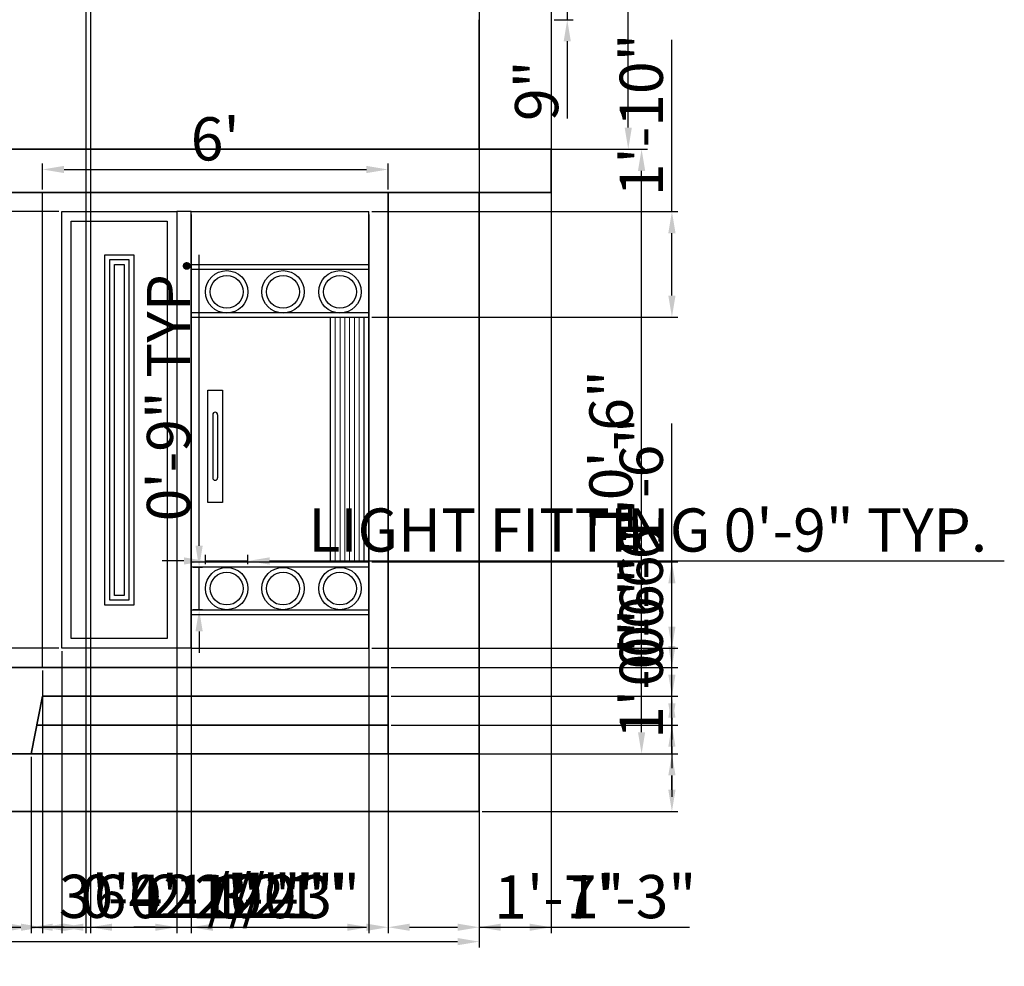
# Model space of a CAD drawing. Units: inches. Extents: x 3297 to 3846, y 520 to 959.
# Tile 3 of 5: x 3641 to 3846, y 520 to 717. Entities that reach past the tile are written whole.
import ezdxf

# ---------------------------------------------------------------- set-up
doc = ezdxf.new("R2010")
doc.units = ezdxf.units.IN
for name, color, linetype, lineweight in [('A-ANNO-DIMS', 2, 'Continuous', 18), ('A-DOOR', 4, 'Continuous', 25), ('A-ELEV', 7, 'Continuous', 35), ('A-ELEV-PATT', 8, 'Continuous', 13)]:
    doc.layers.add(name, color=color, linetype=linetype, lineweight=lineweight)
doc.styles.get("Standard").update_dxf_attribs({"font": 'arial.ttf'})
doc.dimstyles.new('ISO-25', dxfattribs={"dimtxt": 9, "dimasz": 4.5, "dimexe": 1.25, "dimexo": 0.625, "dimtad": 1, "dimdec": 0, "dimlunit": 3, "dimtxsty": 'Standard', "dimcen": 2.5, "dimadec": 0, "dimazin": 0, "dimtfac": 1, "dimtdec": 0, "dimtmove": 0, "dimatfit": 3, "dimfxl": 1, "dimarcsym": 0})

# ---------------------------------------------------------------- blocks, each defined once
blk = doc.blocks.new('*D1')
at = {"layer": 'A-ANNO-DIMS', "color": 0, "lineweight": -2, "transparency": 16777216}
for p, q in [((3737.69, 690.24), (3772.14, 690.24)), ((3770.89, 568.74), (3770.89, 685.74)), ((3737.69, 564.24), (3772.14, 564.24))]:
    blk.add_line(p, q, dxfattribs=at)
at = {"layer": 'A-ANNO-DIMS', "color": 0, "transparency": 16777216}
for points in [[(3770.14, 685.74), (3771.64, 685.74), (3770.89, 690.24)], [(3770.14, 568.74), (3771.64, 568.74), (3770.89, 564.24)]]:
    blk.add_solid(points, dxfattribs=at)
at = {"layer": 'Defpoints', "color": 0, "transparency": 16777216}
for p in [(3737.06, 690.24), (3770.89, 690.24), (3737.06, 564.24)]:
    blk.add_point(p, dxfattribs=at)
at = {"layer": 'A-ANNO-DIMS', "color": 0, "transparency": 16777216, "insert": (3765.67, 627.24), "char_height": 9, "attachment_point": 5, "rotation": 90}
blk.add_mtext('10\'-6"', dxfattribs=at)
blk = doc.blocks.new('*D2')
at = {"layer": 'A-ANNO-DIMS', "color": 0, "lineweight": -2, "transparency": 16777216}
for p, q in [((3752.69, 828.24), (3769.36, 828.24)), ((3768.11, 694.74), (3768.11, 823.74)), ((3752.69, 690.24), (3769.36, 690.24))]:
    blk.add_line(p, q, dxfattribs=at)
at = {"layer": 'A-ANNO-DIMS', "color": 0, "transparency": 16777216}
for points in [[(3767.36, 823.74), (3768.86, 823.74), (3768.11, 828.24)], [(3767.36, 694.74), (3768.86, 694.74), (3768.11, 690.24)]]:
    blk.add_solid(points, dxfattribs=at)
at = {"layer": 'Defpoints', "color": 0, "transparency": 16777216}
for p in [(3752.06, 828.24), (3768.11, 828.24), (3752.06, 690.24)]:
    blk.add_point(p, dxfattribs=at)
at = {"layer": 'A-ANNO-DIMS', "color": 0, "transparency": 16777216, "insert": (3762.89, 759.24), "char_height": 9, "attachment_point": 5, "rotation": 90}
blk.add_mtext('11\'-6"', dxfattribs=at)
blk = doc.blocks.new('*D7')
at = {"layer": 'A-ANNO-DIMS', "color": 0, "lineweight": -2, "transparency": 16777216}
for p, q in [((3332.06, 551.62), (3332.06, 523.84)), ((3737.06, 551.62), (3737.06, 523.84)), ((3336.56, 525.09), (3732.56, 525.09))]:
    blk.add_line(p, q, dxfattribs=at)
at = {"layer": 'A-ANNO-DIMS', "color": 0, "transparency": 16777216}
for points in [[(3336.56, 525.84), (3336.56, 524.34), (3332.06, 525.09)], [(3732.56, 525.84), (3732.56, 524.34), (3737.06, 525.09)]]:
    blk.add_solid(points, dxfattribs=at)
at = {"layer": 'Defpoints', "color": 0, "transparency": 16777216}
for p in [(3332.06, 552.24), (3737.06, 552.24), (3737.06, 525.09)]:
    blk.add_point(p, dxfattribs=at)
at = {"layer": 'A-ANNO-DIMS', "color": 0, "transparency": 16777216, "insert": (3534.56, 530.31), "char_height": 9, "attachment_point": 5}
blk.add_mtext('33\'-9"', dxfattribs=at)
blk = doc.blocks.new('*D11')
at = {"layer": 'A-ANNO-DIMS', "color": 0, "lineweight": -2, "transparency": 16777216}
for p, q in [((3646.06, 681.87), (3646.06, 687.27)), ((3650.56, 686.02), (3713.56, 686.02)), ((3718.06, 681.87), (3718.06, 687.27))]:
    blk.add_line(p, q, dxfattribs=at)
at = {"layer": 'A-ANNO-DIMS', "color": 0, "transparency": 16777216}
for points in [[(3650.56, 686.77), (3650.56, 685.27), (3646.06, 686.02)], [(3713.56, 686.77), (3713.56, 685.27), (3718.06, 686.02)]]:
    blk.add_solid(points, dxfattribs=at)
at = {"layer": 'Defpoints', "color": 0, "transparency": 16777216}
for p in [(3718.06, 686.02), (3646.06, 681.24), (3718.06, 681.24)]:
    blk.add_point(p, dxfattribs=at)
at = {"layer": 'A-ANNO-DIMS', "color": 0, "transparency": 16777216, "insert": (3682.06, 691.24), "char_height": 9, "attachment_point": 5}
blk.add_mtext("6'", dxfattribs=at)
blk = doc.blocks.new('*D17')
at = {"layer": 'A-ANNO-DIMS', "color": 0, "lineweight": -2, "transparency": 16777216}
for p, q in [((3755.4, 730.74), (3755.4, 735.24)), ((3752.69, 726.24), (3756.65, 726.24)), ((3755.4, 726.24), (3755.4, 717.24)), ((3752.69, 717.24), (3756.65, 717.24)), ((3755.4, 712.74), (3755.4, 696.65))]:
    blk.add_line(p, q, dxfattribs=at)
at = {"layer": 'A-ANNO-DIMS', "color": 0, "transparency": 16777216}
for points in [[(3754.65, 730.74), (3756.15, 730.74), (3755.4, 726.24)], [(3754.65, 712.74), (3756.15, 712.74), (3755.4, 717.24)]]:
    blk.add_solid(points, dxfattribs=at)
at = {"layer": 'Defpoints', "color": 0, "transparency": 16777216}
for p in [(3752.06, 726.24), (3752.06, 717.24), (3755.4, 717.24)]:
    blk.add_point(p, dxfattribs=at)
at = {"layer": 'A-ANNO-DIMS', "color": 0, "transparency": 16777216, "insert": (3750.18, 702.44), "char_height": 9, "attachment_point": 5, "rotation": 90}
blk.add_mtext('9"', dxfattribs=at)
blk = doc.blocks.new('LIGHT-ROUND')
for radius in [4.42, 3.42]:
    blk.add_circle((3684.44, 660.52), radius)
blk = doc.blocks.new('*D25')
at = {"layer": 'A-ANNO-DIMS', "color": 0, "lineweight": -2, "transparency": 16777216}
for p, q in [((3680.01, 603.73), (3680.01, 605.68)), ((3688.86, 603.73), (3688.86, 605.68)), ((3675.51, 604.43), (3671.01, 604.43)), ((3680.01, 604.43), (3688.86, 604.43)), ((3693.36, 604.43), (3846.47, 604.43))]:
    blk.add_line(p, q, dxfattribs=at)
at = {"layer": 'A-ANNO-DIMS', "color": 0, "transparency": 16777216}
for points in [[(3675.51, 605.18), (3675.51, 603.68), (3680.01, 604.43)], [(3693.36, 605.18), (3693.36, 603.68), (3688.86, 604.43)]]:
    blk.add_solid(points, dxfattribs=at)
at = {"layer": 'Defpoints', "color": 0, "transparency": 16777216}
for p in [(3688.86, 604.43), (3680.01, 603.1), (3688.86, 603.1)]:
    blk.add_point(p, dxfattribs=at)
at = {"layer": 'A-ANNO-DIMS', "color": 0, "transparency": 16777216, "insert": (3772.17, 609.71), "char_height": 9, "attachment_point": 5}
blk.add_mtext('LIGHT FITTING 0\'-9" TYP.', dxfattribs=at)
blk = doc.blocks.new('*D26')
at = {"layer": 'A-ANNO-DIMS', "color": 0, "lineweight": -2, "transparency": 16777216}
for p, q in [((3678.69, 607.6), (3678.69, 668.21)), ((3679.39, 603.1), (3677.44, 603.1)), ((3678.69, 594.25), (3678.69, 603.1)), ((3679.39, 594.25), (3677.44, 594.25)), ((3678.69, 589.75), (3678.69, 585.25))]:
    blk.add_line(p, q, dxfattribs=at)
at = {"layer": 'A-ANNO-DIMS', "color": 0, "transparency": 16777216}
for points in [[(3677.94, 607.6), (3679.44, 607.6), (3678.69, 603.1)], [(3677.94, 589.75), (3679.44, 589.75), (3678.69, 594.25)]]:
    blk.add_solid(points, dxfattribs=at)
at = {"layer": 'Defpoints', "color": 0, "transparency": 16777216}
for p in [(3678.69, 603.1), (3680.01, 603.1), (3680.01, 594.25)]:
    blk.add_point(p, dxfattribs=at)
at = {"layer": 'A-ANNO-DIMS', "color": 0, "transparency": 16777216, "insert": (3673.47, 640.16), "char_height": 9, "attachment_point": 5, "rotation": 90}
blk.add_mtext('0\'-9" TYP.', dxfattribs=at)
blk = doc.blocks.new('*D41')
at = {"layer": 'A-ANNO-DIMS', "color": 0, "lineweight": -2, "transparency": 16777216}
for p, q in [((3655.06, 882.62), (3655.06, 526.84)), ((3656.06, 882.62), (3656.06, 526.84)), ((3650.56, 528.09), (3646.06, 528.09)), ((3655.06, 528.09), (3656.06, 528.09)), ((3660.56, 528.09), (3690.24, 528.09))]:
    blk.add_line(p, q, dxfattribs=at)
at = {"layer": 'A-ANNO-DIMS', "color": 0, "transparency": 16777216}
for points in [[(3650.56, 528.84), (3650.56, 527.34), (3655.06, 528.09)], [(3660.56, 528.84), (3660.56, 527.34), (3656.06, 528.09)]]:
    blk.add_solid(points, dxfattribs=at)
at = {"layer": 'Defpoints', "color": 0, "transparency": 16777216}
for p in [(3655.06, 883.24), (3656.06, 883.24), (3656.06, 528.09)]:
    blk.add_point(p, dxfattribs=at)
at = {"layer": 'A-ANNO-DIMS', "color": 0, "transparency": 16777216, "insert": (3677.65, 533.31), "char_height": 9, "attachment_point": 5}
blk.add_mtext('0\'-1"', dxfattribs=at)
blk = doc.blocks.new('*D45')
at = {"layer": 'A-ANNO-DIMS', "color": 0, "lineweight": -2, "transparency": 16777216}
for p, q in [((3737.06, 816.62), (3737.06, 526.84)), ((3752.06, 816.62), (3752.06, 526.84)), ((3741.56, 528.09), (3747.56, 528.09)), ((3752.06, 528.09), (3780.89, 528.09))]:
    blk.add_line(p, q, dxfattribs=at)
at = {"layer": 'A-ANNO-DIMS', "color": 0, "transparency": 16777216}
for points in [[(3741.56, 528.84), (3741.56, 527.34), (3737.06, 528.09)], [(3747.56, 528.84), (3747.56, 527.34), (3752.06, 528.09)]]:
    blk.add_solid(points, dxfattribs=at)
at = {"layer": 'Defpoints', "color": 0, "transparency": 16777216}
for p in [(3737.06, 817.24), (3752.06, 817.24), (3752.06, 528.09)]:
    blk.add_point(p, dxfattribs=at)
at = {"layer": 'A-ANNO-DIMS', "color": 0, "transparency": 16777216, "insert": (3768.73, 533.31), "char_height": 9, "attachment_point": 5}
blk.add_mtext('1\'-3"', dxfattribs=at)
blk = doc.blocks.new('*D46')
at = {"layer": 'A-ANNO-DIMS', "color": 0, "lineweight": -2, "transparency": 16777216}
for p, q in [((3777.21, 564.24), (3777.21, 593.07)), ((3737.69, 564.24), (3778.46, 564.24)), ((3777.21, 556.74), (3777.21, 559.74)), ((3737.69, 552.24), (3778.46, 552.24))]:
    blk.add_line(p, q, dxfattribs=at)
at = {"layer": 'A-ANNO-DIMS', "color": 0, "transparency": 16777216}
for points in [[(3776.46, 559.74), (3777.96, 559.74), (3777.21, 564.24)], [(3776.46, 556.74), (3777.96, 556.74), (3777.21, 552.24)]]:
    blk.add_solid(points, dxfattribs=at)
at = {"layer": 'Defpoints', "color": 0, "transparency": 16777216}
for p in [(3737.06, 564.24), (3777.21, 564.24), (3737.06, 552.24)]:
    blk.add_point(p, dxfattribs=at)
at = {"layer": 'A-ANNO-DIMS', "color": 0, "transparency": 16777216, "insert": (3771.99, 580.9), "char_height": 9, "attachment_point": 5, "rotation": 90}
blk.add_mtext('1\'-0"', dxfattribs=at)
blk = doc.blocks.new('*D47')
at = {"layer": 'A-ANNO-DIMS', "color": 0, "lineweight": -2, "transparency": 16777216}
for p, q in [((3777.21, 574.74), (3777.21, 604.42)), ((3718.69, 570.24), (3778.46, 570.24)), ((3777.21, 564.24), (3777.21, 570.24)), ((3718.69, 564.24), (3778.46, 564.24)), ((3777.21, 559.74), (3777.21, 555.24))]:
    blk.add_line(p, q, dxfattribs=at)
at = {"layer": 'A-ANNO-DIMS', "color": 0, "transparency": 16777216}
for points in [[(3776.46, 574.74), (3777.96, 574.74), (3777.21, 570.24)], [(3776.46, 559.74), (3777.96, 559.74), (3777.21, 564.24)]]:
    blk.add_solid(points, dxfattribs=at)
at = {"layer": 'Defpoints', "color": 0, "transparency": 16777216}
for p in [(3718.06, 570.24), (3777.21, 570.24), (3718.06, 564.24)]:
    blk.add_point(p, dxfattribs=at)
at = {"layer": 'A-ANNO-DIMS', "color": 0, "transparency": 16777216, "insert": (3771.99, 591.83), "char_height": 9, "attachment_point": 5, "rotation": 90}
blk.add_mtext('0\'-6"', dxfattribs=at)
blk = doc.blocks.new('*D48')
at = {"layer": 'A-ANNO-DIMS', "color": 0, "lineweight": -2, "transparency": 16777216}
for p, q in [((3777.21, 580.74), (3777.21, 610.42)), ((3718.69, 576.24), (3778.46, 576.24)), ((3777.21, 570.24), (3777.21, 576.24)), ((3718.69, 570.24), (3778.46, 570.24)), ((3777.21, 565.74), (3777.21, 561.24))]:
    blk.add_line(p, q, dxfattribs=at)
at = {"layer": 'A-ANNO-DIMS', "color": 0, "transparency": 16777216}
for points in [[(3776.46, 580.74), (3777.96, 580.74), (3777.21, 576.24)], [(3776.46, 565.74), (3777.96, 565.74), (3777.21, 570.24)]]:
    blk.add_solid(points, dxfattribs=at)
at = {"layer": 'Defpoints', "color": 0, "transparency": 16777216}
for p in [(3718.06, 576.24), (3777.21, 576.24), (3718.06, 570.24)]:
    blk.add_point(p, dxfattribs=at)
at = {"layer": 'A-ANNO-DIMS', "color": 0, "transparency": 16777216, "insert": (3771.99, 597.83), "char_height": 9, "attachment_point": 5, "rotation": 90}
blk.add_mtext('0\'-6"', dxfattribs=at)
blk = doc.blocks.new('*D49')
at = {"layer": 'A-ANNO-DIMS', "color": 0, "lineweight": -2, "transparency": 16777216}
for p, q in [((3777.21, 586.74), (3777.21, 616.42)), ((3718.69, 582.24), (3778.46, 582.24)), ((3777.21, 576.24), (3777.21, 582.24)), ((3718.69, 576.24), (3778.46, 576.24)), ((3777.21, 571.74), (3777.21, 567.24))]:
    blk.add_line(p, q, dxfattribs=at)
at = {"layer": 'A-ANNO-DIMS', "color": 0, "transparency": 16777216}
for points in [[(3776.46, 586.74), (3777.96, 586.74), (3777.21, 582.24)], [(3776.46, 571.74), (3777.96, 571.74), (3777.21, 576.24)]]:
    blk.add_solid(points, dxfattribs=at)
at = {"layer": 'Defpoints', "color": 0, "transparency": 16777216}
for p in [(3718.06, 582.24), (3777.21, 582.24), (3718.06, 576.24)]:
    blk.add_point(p, dxfattribs=at)
at = {"layer": 'A-ANNO-DIMS', "color": 0, "transparency": 16777216, "insert": (3771.99, 603.83), "char_height": 9, "attachment_point": 5, "rotation": 90}
blk.add_mtext('0\'-6"', dxfattribs=at)
blk = doc.blocks.new('*D50')
at = {"layer": 'A-ANNO-DIMS', "color": 0, "lineweight": -2, "transparency": 16777216}
for p, q in [((3643.69, 563.62), (3643.69, 526.84)), ((3718.06, 563.62), (3718.06, 526.84)), ((3648.19, 528.09), (3713.56, 528.09))]:
    blk.add_line(p, q, dxfattribs=at)
at = {"layer": 'A-ANNO-DIMS', "color": 0, "transparency": 16777216}
for points in [[(3648.19, 528.84), (3648.19, 527.34), (3643.69, 528.09)], [(3713.56, 528.84), (3713.56, 527.34), (3718.06, 528.09)]]:
    blk.add_solid(points, dxfattribs=at)
at = {"layer": 'Defpoints', "color": 0, "transparency": 16777216}
for p in [(3643.69, 564.24), (3718.06, 564.24), (3718.06, 528.09)]:
    blk.add_point(p, dxfattribs=at)
at = {"layer": 'A-ANNO-DIMS', "color": 0, "transparency": 16777216, "insert": (3680.88, 533.37), "char_height": 9, "attachment_point": 5}
blk.add_mtext('6\'-2 1/2"', dxfattribs=at)
blk = doc.blocks.new('*D51')
at = {"layer": 'A-ANNO-DIMS', "color": 0, "lineweight": -2, "transparency": 16777216}
for p, q in [((3646.06, 575.62), (3646.06, 526.84)), ((3643.69, 563.62), (3643.69, 526.84)), ((3639.19, 528.09), (3634.69, 528.09)), ((3643.69, 528.09), (3646.06, 528.09)), ((3650.56, 528.09), (3701.21, 528.09))]:
    blk.add_line(p, q, dxfattribs=at)
at = {"layer": 'A-ANNO-DIMS', "color": 0, "transparency": 16777216}
for points in [[(3639.19, 528.84), (3639.19, 527.34), (3643.69, 528.09)], [(3650.56, 528.84), (3650.56, 527.34), (3646.06, 528.09)]]:
    blk.add_solid(points, dxfattribs=at)
at = {"layer": 'Defpoints', "color": 0, "transparency": 16777216}
for p in [(3646.06, 576.24), (3643.69, 564.24), (3646.06, 528.09)]:
    blk.add_point(p, dxfattribs=at)
at = {"layer": 'A-ANNO-DIMS', "color": 0, "transparency": 16777216, "insert": (3678.14, 533.37), "char_height": 9, "attachment_point": 5}
blk.add_mtext('0\'-2 1/2"', dxfattribs=at)
blk = doc.blocks.new('*D53')
at = {"layer": 'A-ANNO-DIMS', "color": 0, "lineweight": -2, "transparency": 16777216}
for p, q in [((3605.76, 599.62), (3605.76, 526.84)), ((3646.06, 581.62), (3646.06, 526.84)), ((3610.26, 528.09), (3641.56, 528.09)), ((3646.06, 528.09), (3696.7, 528.09))]:
    blk.add_line(p, q, dxfattribs=at)
at = {"layer": 'A-ANNO-DIMS', "color": 0, "transparency": 16777216}
for points in [[(3610.26, 528.84), (3610.26, 527.34), (3605.76, 528.09)], [(3641.56, 528.84), (3641.56, 527.34), (3646.06, 528.09)]]:
    blk.add_solid(points, dxfattribs=at)
at = {"layer": 'Defpoints', "color": 0, "transparency": 16777216}
for p in [(3605.76, 600.24), (3646.06, 582.24), (3646.06, 528.09)]:
    blk.add_point(p, dxfattribs=at)
at = {"layer": 'A-ANNO-DIMS', "color": 0, "transparency": 16777216, "insert": (3673.63, 533.37), "char_height": 9, "attachment_point": 5}
blk.add_mtext('3\'-4 1/2"', dxfattribs=at)
blk = doc.blocks.new('*D54')
at = {"layer": 'A-ANNO-DIMS', "color": 0, "lineweight": -2, "transparency": 16777216}
for p, q in [((3718.06, 581.62), (3718.06, 526.84)), ((3737.06, 563.62), (3737.06, 526.84)), ((3722.56, 528.09), (3732.56, 528.09)), ((3737.06, 528.09), (3765.89, 528.09))]:
    blk.add_line(p, q, dxfattribs=at)
at = {"layer": 'A-ANNO-DIMS', "color": 0, "transparency": 16777216}
for points in [[(3722.56, 528.84), (3722.56, 527.34), (3718.06, 528.09)], [(3732.56, 528.84), (3732.56, 527.34), (3737.06, 528.09)]]:
    blk.add_solid(points, dxfattribs=at)
at = {"layer": 'Defpoints', "color": 0, "transparency": 16777216}
for p in [(3718.06, 582.24), (3737.06, 564.24), (3737.06, 528.09)]:
    blk.add_point(p, dxfattribs=at)
at = {"layer": 'A-ANNO-DIMS', "color": 0, "transparency": 16777216, "insert": (3753.73, 533.23), "char_height": 9, "attachment_point": 5}
blk.add_mtext('1\'-7"', dxfattribs=at)
blk = doc.blocks.new('*D57')
at = {"layer": 'A-ANNO-DIMS', "color": 0, "lineweight": -2, "transparency": 16777216}
for p, q in [((3645.44, 681.24), (3306.66, 681.24)), ((3307.91, 586.74), (3307.91, 676.74)), ((3645.44, 582.24), (3306.66, 582.24))]:
    blk.add_line(p, q, dxfattribs=at)
at = {"layer": 'A-ANNO-DIMS', "color": 0, "transparency": 16777216}
for points in [[(3307.16, 676.74), (3308.66, 676.74), (3307.91, 681.24)], [(3307.16, 586.74), (3308.66, 586.74), (3307.91, 582.24)]]:
    blk.add_solid(points, dxfattribs=at)
at = {"layer": 'Defpoints', "color": 0, "transparency": 16777216}
for p in [(3307.91, 681.24), (3646.06, 681.24), (3646.06, 582.24)]:
    blk.add_point(p, dxfattribs=at)
at = {"layer": 'A-ANNO-DIMS', "color": 0, "transparency": 16777216, "insert": (3302.69, 631.74), "char_height": 9, "attachment_point": 5, "rotation": 90}
blk.add_mtext('8\'-3"', dxfattribs=at)
blk = doc.blocks.new('*D58')
at = {"layer": 'A-ANNO-DIMS', "color": 0, "lineweight": -2, "transparency": 16777216}
for p, q in [((3650.06, 585.62), (3650.06, 526.84)), ((3674.06, 585.62), (3674.06, 526.84)), ((3654.56, 528.09), (3669.56, 528.09)), ((3674.06, 528.09), (3703.89, 528.09))]:
    blk.add_line(p, q, dxfattribs=at)
at = {"layer": 'A-ANNO-DIMS', "color": 0, "transparency": 16777216}
for points in [[(3654.56, 528.84), (3654.56, 527.34), (3650.06, 528.09)], [(3669.56, 528.84), (3669.56, 527.34), (3674.06, 528.09)]]:
    blk.add_solid(points, dxfattribs=at)
at = {"layer": 'Defpoints', "color": 0, "transparency": 16777216}
for p in [(3650.06, 586.24), (3674.06, 586.24), (3674.06, 528.09)]:
    blk.add_point(p, dxfattribs=at)
at = {"layer": 'A-ANNO-DIMS', "color": 0, "transparency": 16777216, "insert": (3691.23, 533.31), "char_height": 9, "attachment_point": 5}
blk.add_mtext('2\'-0"', dxfattribs=at)
blk = doc.blocks.new('*D59')
at = {"layer": 'A-ANNO-DIMS', "color": 0, "lineweight": -2, "transparency": 16777216}
for p, q in [((3649.439671, 677.241209), (3306.664671, 677.241209)), ((3307.914671, 590.741209), (3307.914671, 672.741209)), ((3649.439671, 586.241209), (3306.664671, 586.241209))]:
    blk.add_line(p, q, dxfattribs=at)
at = {"layer": 'A-ANNO-DIMS', "color": 0, "transparency": 16777216}
for points in [[(3307.164671, 672.741209), (3308.664671, 672.741209), (3307.914671, 677.241209)], [(3307.164671, 590.741209), (3308.664671, 590.741209), (3307.914671, 586.241209)]]:
    blk.add_solid(points, dxfattribs=at)
at = {"layer": 'Defpoints', "color": 0, "transparency": 16777216}
for p in [(3307.914671, 677.241209), (3650.064671, 677.241209), (3650.064671, 586.241209)]:
    blk.add_point(p, dxfattribs=at)
at = {"layer": 'A-ANNO-DIMS', "color": 0, "transparency": 16777216, "insert": (3302.789671, 631.741209), "char_height": 9, "attachment_point": 5, "rotation": 90}
blk.add_mtext('7\'-7"', dxfattribs=at)
blk = doc.blocks.new('*D60')
at = {"layer": 'A-ANNO-DIMS', "color": 0, "lineweight": -2, "transparency": 16777216}
for p, q in [((3674.06, 676.62), (3674.06, 526.84)), ((3677.06, 676.62), (3677.06, 526.84)), ((3669.56, 528.09), (3665.06, 528.09)), ((3674.06, 528.09), (3677.06, 528.09)), ((3681.56, 528.09), (3711.24, 528.09))]:
    blk.add_line(p, q, dxfattribs=at)
at = {"layer": 'A-ANNO-DIMS', "color": 0, "transparency": 16777216}
for points in [[(3669.56, 528.84), (3669.56, 527.34), (3674.06, 528.09)], [(3681.56, 528.84), (3681.56, 527.34), (3677.06, 528.09)]]:
    blk.add_solid(points, dxfattribs=at)
at = {"layer": 'Defpoints', "color": 0, "transparency": 16777216}
for p in [(3674.06, 677.24), (3677.06, 677.24), (3677.06, 528.09)]:
    blk.add_point(p, dxfattribs=at)
at = {"layer": 'A-ANNO-DIMS', "color": 0, "transparency": 16777216, "insert": (3698.65, 533.31), "char_height": 9, "attachment_point": 5}
blk.add_mtext('0\'-3"', dxfattribs=at)
blk = doc.blocks.new('*D61')
at = {"layer": 'A-ANNO-DIMS', "color": 0, "lineweight": -2, "transparency": 16777216}
for p, q in [((3677.06, 676.62), (3677.06, 526.84)), ((3714.06, 676.62), (3714.06, 526.84)), ((3681.56, 528.09), (3709.56, 528.09))]:
    blk.add_line(p, q, dxfattribs=at)
at = {"layer": 'A-ANNO-DIMS', "color": 0, "transparency": 16777216}
for points in [[(3681.56, 528.84), (3681.56, 527.34), (3677.06, 528.09)], [(3709.56, 528.84), (3709.56, 527.34), (3714.06, 528.09)]]:
    blk.add_solid(points, dxfattribs=at)
at = {"layer": 'Defpoints', "color": 0, "transparency": 16777216}
for p in [(3677.06, 677.24), (3714.06, 677.24), (3714.06, 528.09)]:
    blk.add_point(p, dxfattribs=at)
at = {"layer": 'A-ANNO-DIMS', "color": 0, "transparency": 16777216, "insert": (3695.56, 533.31), "char_height": 9, "attachment_point": 5}
blk.add_mtext('3\'-1"', dxfattribs=at)
blk = doc.blocks.new('*D62')
at = {"layer": 'A-ANNO-DIMS', "color": 0, "lineweight": -2, "transparency": 16777216}
for p, q in [((3777.21, 677.24), (3777.21, 713.06)), ((3714.69, 677.24), (3778.46, 677.24)), ((3777.21, 659.74), (3777.21, 672.74)), ((3714.69, 655.24), (3778.46, 655.24))]:
    blk.add_line(p, q, dxfattribs=at)
at = {"layer": 'A-ANNO-DIMS', "color": 0, "transparency": 16777216}
for points in [[(3776.46, 672.74), (3777.96, 672.74), (3777.21, 677.24)], [(3776.46, 659.74), (3777.96, 659.74), (3777.21, 655.24)]]:
    blk.add_solid(points, dxfattribs=at)
at = {"layer": 'Defpoints', "color": 0, "transparency": 16777216}
for p in [(3714.06, 677.24), (3777.21, 677.24), (3714.06, 655.24)]:
    blk.add_point(p, dxfattribs=at)
at = {"layer": 'A-ANNO-DIMS', "color": 0, "transparency": 16777216, "insert": (3771.99, 697.4), "char_height": 9, "attachment_point": 5, "rotation": 90}
blk.add_mtext('1\'-10"', dxfattribs=at)
blk = doc.blocks.new('*D63')
at = {"layer": 'A-ANNO-DIMS', "color": 0, "lineweight": -2, "transparency": 16777216}
for p, q in [((3777.21, 604.24), (3777.21, 633.07)), ((3714.69, 604.24), (3778.46, 604.24)), ((3777.21, 590.74), (3777.21, 599.74)), ((3714.69, 586.24), (3778.46, 586.24))]:
    blk.add_line(p, q, dxfattribs=at)
at = {"layer": 'A-ANNO-DIMS', "color": 0, "transparency": 16777216}
for points in [[(3776.46, 599.74), (3777.96, 599.74), (3777.21, 604.24)], [(3776.46, 590.74), (3777.96, 590.74), (3777.21, 586.24)]]:
    blk.add_solid(points, dxfattribs=at)
at = {"layer": 'Defpoints', "color": 0, "transparency": 16777216}
for p in [(3714.06, 604.24), (3777.21, 604.24), (3714.06, 586.24)]:
    blk.add_point(p, dxfattribs=at)
at = {"layer": 'A-ANNO-DIMS', "color": 0, "transparency": 16777216, "insert": (3771.99, 620.9), "char_height": 9, "attachment_point": 5, "rotation": 90}
blk.add_mtext('1\'-6"', dxfattribs=at)

msp = doc.modelspace()

# ---------------------------------------------------------------- linework, layer by layer
at = {"layer": 'A-DOOR'}
for p, q in [((3646.06, 582.24), (3646.06, 681.24)), ((3677.06, 677.24), (3674.06, 677.24)), ((3677.06, 586.24), (3677.06, 677.24)), ((3677.06, 677.24), (3714.06, 677.24)), ((3714.06, 586.24), (3714.06, 677.24)), ((3677.06, 666.24), (3714.06, 666.24)), ((3677.06, 665.24), (3714.06, 665.24)), ((3677.06, 656.24), (3714.06, 656.24)), ((3677.06, 655.24), (3714.06, 655.24)), ((3706.06, 604.24), (3706.06, 655.24)), ((3713.06, 604.24), (3713.06, 655.24)), ((3680.54, 640.04), (3683.54, 640.04)), ((3680.54, 616.64), (3680.54, 640.04)), ((3683.54, 640.04), (3683.54, 616.64)), ((3681.54, 634.92), (3681.54, 621.76)), ((3682.54, 634.92), (3682.54, 621.76)), ((3683.54, 616.64), (3680.54, 616.64)), ((3677.06, 604.24), (3714.06, 604.24)), ((3677.06, 603.24), (3714.06, 603.24)), ((3677.06, 594.24), (3714.06, 594.24)), ((3677.06, 593.24), (3714.06, 593.24)), ((3677.06, 586.24), (3674.06, 586.24)), ((3677.06, 586.24), (3714.06, 586.24))]:
    msp.add_line(p, q, dxfattribs=at)
for points in [[(3650.06, 586.24), (3650.06, 677.24), (3674.06, 677.24), (3674.06, 586.24)], [(3652.06, 588.24), (3652.06, 675.24), (3672.06, 675.24), (3672.06, 588.24)], [(3659.06, 595.24), (3659.06, 668.24), (3665.06, 668.24), (3665.06, 595.24)], [(3660.06, 596.24), (3660.06, 667.24), (3664.06, 667.24), (3664.06, 596.24)], [(3661.06, 597.24), (3661.06, 666.24), (3663.06, 666.24), (3663.06, 597.24)]]:
    msp.add_lwpolyline(points, close=True, dxfattribs=at)
for centre, start, end in [((3682.04, 634.92), 0, 180), ((3682.04, 621.76), 180, 0)]:
    msp.add_arc(centre, 0.5, start, end, dxfattribs=at)
at = {"layer": 'A-ELEV'}
for p, q in [((3737.06, 690.24), (3737.06, 717.24)), ((3488.06, 690.24), (3752.06, 690.24)), ((3752.06, 690.24), (3752.06, 681.24)), ((3506.06, 681.24), (3752.06, 681.24)), ((3718.06, 564.24), (3718.06, 681.24)), ((3737.06, 552.24), (3737.06, 681.24)), ((3512.06, 582.24), (3718.06, 582.24)), ((3646.06, 576.24), (3643.69, 564.24)), ((3646.06, 576.24), (3718.06, 576.24)), ((3644.88, 570.24), (3718.06, 570.24)), ((3512.06, 564.24), (3737.06, 564.24)), ((3332.06, 552.24), (3737.06, 552.24))]:
    msp.add_line(p, q, dxfattribs=at)
at = {"layer": 'A-ELEV-PATT'}
for p, q in [((3707.06, 604.24), (3707.06, 655.24)), ((3708.06, 604.24), (3708.06, 655.24)), ((3709.06, 604.24), (3709.06, 655.24)), ((3710.06, 604.24), (3710.06, 655.24)), ((3711.06, 604.24), (3711.06, 655.24)), ((3712.06, 604.24), (3712.06, 655.24))]:
    msp.add_line(p, q, dxfattribs=at)

# ---------------------------------------------------------------- block references
at = {"layer": 'A-DOOR'}
for p in [(0, 0), (11.74, 0), (23.6, 0), (0, -61.84), (11.74, -61.84), (23.6, -61.84)]:
    msp.add_blockref('LIGHT-ROUND', p, dxfattribs=at)

# ---------------------------------------------------------------- dimensions: what is measured, and where the dimension line sits
at = {"layer": 'A-ANNO-DIMS'}
for base, p1, p2, override, picture, middle in [((3656.06, 528.09), (3655.06, 883.24), (3656.06, 883.24), {"dimdec": 1, "dimlfac": 1, "dimrnd": 0, "dimzin": 1, "dimdsep": 46, "dimlunit": 4, "dimfrac": 2}, '*D41', (3677.65, 533.31)), ((3752.06, 528.09), (3737.06, 817.24), (3752.06, 817.24), {"dimdec": 1, "dimlfac": 1, "dimrnd": 0, "dimzin": 1, "dimdsep": 46, "dimlunit": 4, "dimfrac": 2}, '*D45', (3768.73, 533.31)), ((3718.06, 686.02), (3646.06, 681.24), (3718.06, 681.24), {"dimclrd": 0, "dimclre": 0, "dimclrt": 0}, '*D11', (3682.06, 691.24)), ((3677.06, 528.09), (3674.06, 677.24), (3677.06, 677.24), {"dimdec": 1, "dimlfac": 1, "dimrnd": 0, "dimzin": 1, "dimdsep": 46, "dimlunit": 4, "dimfrac": 2}, '*D60', (3698.65, 533.31)), ((3714.06, 528.09), (3677.06, 677.24), (3714.06, 677.24), {"dimdec": 1, "dimlfac": 1, "dimrnd": 0, "dimzin": 1, "dimdsep": 46, "dimlunit": 4, "dimfrac": 2}, '*D61', (3695.56, 533.31)), ((3646.06, 528.09), (3605.76, 600.24), (3646.06, 582.24), {"dimdec": 1, "dimlfac": 1, "dimrnd": 0, "dimzin": 1, "dimdsep": 46, "dimlunit": 4, "dimfrac": 2}, '*D53', (3673.63, 533.37)), ((3674.06, 528.09), (3650.06, 586.24), (3674.06, 586.24), {"dimdec": 1, "dimlfac": 1, "dimrnd": 0, "dimzin": 1, "dimdsep": 46, "dimlunit": 4, "dimfrac": 2}, '*D58', (3691.23, 533.31)), ((3737.06, 528.09), (3718.06, 582.24), (3737.06, 564.24), {"dimdec": 1, "dimlfac": 1, "dimrnd": 0, "dimzin": 1, "dimdsep": 46, "dimlunit": 4, "dimfrac": 2}, '*D54', (3753.73, 533.23)), ((3646.06, 528.09), (3643.69, 564.24), (3646.06, 576.24), {"dimdec": 1, "dimlfac": 1, "dimrnd": 0, "dimzin": 1, "dimdsep": 46, "dimlunit": 4, "dimfrac": 2}, '*D51', (3678.14, 533.37)), ((3718.06, 528.09), (3643.69, 564.24), (3718.06, 564.24), {"dimdec": 1, "dimlfac": 1, "dimrnd": 0, "dimzin": 1, "dimdsep": 46, "dimlunit": 4, "dimfrac": 2}, '*D50', (3680.88, 533.37)), ((3737.06, 525.09), (3332.06, 552.24), (3737.06, 552.24), {"dimclrd": 0, "dimclre": 0, "dimclrt": 0}, '*D7', (3534.56, 530.31))]:
    dim = msp.add_linear_dim(base=base, p1=p1, p2=p2, dimstyle='ISO-25', override=override, dxfattribs=at)
    dim.commit()
    dim.dimension.update_dxf_attribs({"geometry": picture, "text_midpoint": middle})
for base, p1, p2, override, picture, middle in [((3768.11, 828.24), (3752.06, 690.24), (3752.06, 828.24), {"dimclrd": 0, "dimclre": 0, "dimclrt": 0}, '*D2', (3762.89, 759.24)), ((3755.4, 717.24), (3752.06, 726.24), (3752.06, 717.24), {"dimclrd": 0, "dimclre": 0, "dimclrt": 0}, '*D17', (3750.18, 702.44)), ((3777.21, 677.24), (3714.06, 655.24), (3714.06, 677.24), {"dimdec": 1, "dimlfac": 1, "dimrnd": 0, "dimzin": 1, "dimdsep": 46, "dimlunit": 4, "dimfrac": 2}, '*D62', (3771.99, 697.4)), ((3770.89, 690.24), (3737.06, 564.24), (3737.06, 690.24), {"dimclrd": 0, "dimclre": 0, "dimclrt": 0}, '*D1', (3765.67, 627.24)), ((3307.91, 681.24), (3646.06, 582.24), (3646.06, 681.24), {"dimdec": 1, "dimlfac": 1, "dimrnd": 0, "dimzin": 1, "dimdsep": 46, "dimlunit": 4, "dimfrac": 2}, '*D57', (3302.69, 631.74)), ((3307.91, 677.24), (3650.06, 586.24), (3650.06, 677.24), {"dimdec": 1, "dimlfac": 1, "dimrnd": 0, "dimzin": 1, "dimdsep": 46, "dimlunit": 4, "dimfrac": 2}, '*D59', (3302.79, 631.74)), ((3777.21, 604.24), (3714.06, 586.24), (3714.06, 604.24), {"dimdec": 1, "dimlfac": 1, "dimrnd": 0, "dimzin": 1, "dimdsep": 46, "dimlunit": 4, "dimfrac": 2}, '*D63', (3771.99, 620.9)), ((3777.21, 582.24), (3718.06, 576.24), (3718.06, 582.24), {"dimdec": 1, "dimlfac": 1, "dimrnd": 0, "dimzin": 1, "dimdsep": 46, "dimlunit": 4, "dimfrac": 2}, '*D49', (3771.99, 603.83)), ((3777.21, 576.24), (3718.06, 570.24), (3718.06, 576.24), {"dimdec": 1, "dimlfac": 1, "dimrnd": 0, "dimzin": 1, "dimdsep": 46, "dimlunit": 4, "dimfrac": 2}, '*D48', (3771.99, 597.83)), ((3777.21, 570.24), (3718.06, 564.24), (3718.06, 570.24), {"dimdec": 1, "dimlfac": 1, "dimrnd": 0, "dimzin": 1, "dimdsep": 46, "dimlunit": 4, "dimfrac": 2}, '*D47', (3771.99, 591.83)), ((3777.21, 564.24), (3737.06, 552.24), (3737.06, 564.24), {"dimdec": 1, "dimlfac": 1, "dimrnd": 0, "dimzin": 1, "dimdsep": 46, "dimlunit": 4, "dimfrac": 2}, '*D46', (3771.99, 580.9))]:
    dim = msp.add_linear_dim(base=base, p1=p1, p2=p2, angle=90, dimstyle='ISO-25', override=override, dxfattribs=at)
    dim.commit()
    dim.dimension.update_dxf_attribs({"geometry": picture, "text_midpoint": middle})
dim = msp.add_linear_dim(base=(3678.6868, 603.1014), p1=(3680.0142, 594.2517), p2=(3680.0142, 603.1014), angle=90, text='<> TYP.', dimstyle='ISO-25', override={"dimdec": 1, "dimrnd": 0, "dimzin": 1, "dimlunit": 4, "dimfrac": 2}, dxfattribs=at)
dim.commit()
dim.dimension.update_dxf_attribs({"geometry": '*D26', "text_midpoint": (3673.4666, 640.1562)})
dim = msp.add_linear_dim(base=(3688.8639, 604.4289), p1=(3680.0142, 603.1014), p2=(3688.8639, 603.1014), text='LIGHT FITTING <> TYP.', dimstyle='ISO-25', override={"dimdec": 1, "dimrnd": 0, "dimzin": 1, "dimlunit": 4, "dimfrac": 2}, dxfattribs=at)
dim.commit()
dim.dimension.update_dxf_attribs({"geometry": '*D25', "text_midpoint": (3772.168, 609.7074)})

doc.saveas('drawing.dxf')
